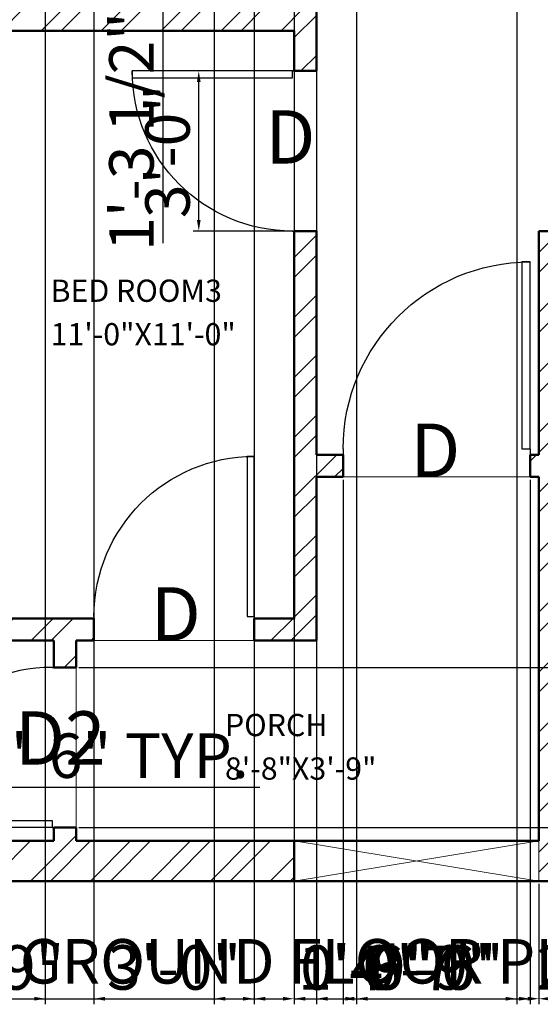
# Model space of a CAD drawing. Units: inches. Extents: x 3824 to 4289, y 1731 to 2259.
# Tile 2 of 5: x 3952 to 4069, y 1731 to 1952. Entities that reach past the tile are written whole.
import ezdxf

# ---------------------------------------------------------------- set-up
doc = ezdxf.new("R2010")
doc.units = ezdxf.units.IN
for name, color, linetype, lineweight in [('A-ANNO-DIMS', 2, 'Continuous', 18), ('A-ANNO-TEXT', 2, 'Continuous', 18), ('A-ANNO-TITL', 2, 'Continuous', 25), ('A-AREA-IDEN', 2, 'Continuous', 18), ('A-FLOR-THRS', 8, 'Continuous', 18), ('DOOR', 6, 'Continuous', 25), ('WALL', 20, 'Continuous', 50)]:
    doc.layers.add(name, color=color, linetype=linetype, lineweight=lineweight)
doc.layers.add('A-WALL-PATT', color=251, linetype='Continuous', lineweight=13, true_color=0x636466)
doc.styles.get("Standard").update_dxf_attribs({"font": 'arial.ttf'})
doc.dimstyles.new('ISO-25', dxfattribs={"dimtxt": 10, "dimasz": 2.5, "dimexe": 1.25, "dimexo": 0.625, "dimtad": 1, "dimdec": 1, "dimlunit": 3, "dimtxsty": 'Standard', "dimcen": 2.5, "dimadec": 0, "dimazin": 0, "dimtfac": 1, "dimtdec": 1, "dimtmove": 0, "dimatfit": 3, "dimfxl": 1, "dimarcsym": 0})

# ---------------------------------------------------------------- blocks, each defined once
blk = doc.blocks.new('*U2')
for p, q in [((0, 0), (0, -6)), ((40, 0), (40, -6))]:
    blk.add_line(p, q)
blk.add_lwpolyline([(0, 0), (0, 40), (1.75, 40), (1.75, 0)], close=True)
blk.add_arc((0, 0), 40, 0, 90)
blk = doc.blocks.new('*D16')
at = {"layer": 'A-ANNO-DIMS', "color": 0, "lineweight": -2, "transparency": 16777216}
for p, q in [((3883.53, 1783.56), (3883.53, 1778.43)), ((3913.57, 1783.56), (3913.57, 1778.43)), ((3886.03, 1779.68), (3911.07, 1779.68)), ((3913.57, 1779.68), (4005.84, 1779.68))]:
    blk.add_line(p, q, dxfattribs=at)
at = {"layer": 'A-ANNO-DIMS', "color": 0, "transparency": 16777216}
for points in [[(3886.03, 1780.1), (3886.03, 1779.27), (3883.53, 1779.68)], [(3911.07, 1780.1), (3911.07, 1779.27), (3913.57, 1779.68)]]:
    blk.add_solid(points, dxfattribs=at)
at = {"layer": 'Defpoints', "color": 0, "transparency": 16777216}
for p in [(3883.53, 1784.19), (3913.57, 1784.19), (3913.57, 1779.68)]:
    blk.add_point(p, dxfattribs=at)
at = {"layer": 'A-ANNO-DIMS', "color": 0, "transparency": 16777216, "insert": (3960.95, 1785.48), "char_height": 10, "attachment_point": 5}
blk.add_mtext('WC 2\'-6" TYP.', dxfattribs=at)
blk = doc.blocks.new('*D38')
at = {"layer": 'A-ANNO-DIMS', "color": 0, "lineweight": -2, "transparency": 16777216}
for p, q in [((3872.55, 1757.99), (3872.55, 1730.92)), ((4013.55, 1757.99), (4013.55, 1730.92)), ((3875.05, 1732.17), (4011.05, 1732.17))]:
    blk.add_line(p, q, dxfattribs=at)
at = {"layer": 'A-ANNO-DIMS', "color": 0, "transparency": 16777216}
for points in [[(3875.05, 1732.59), (3875.05, 1731.75), (3872.55, 1732.17)], [(4011.05, 1732.59), (4011.05, 1731.75), (4013.55, 1732.17)]]:
    blk.add_solid(points, dxfattribs=at)
at = {"layer": 'Defpoints', "color": 0, "transparency": 16777216}
for p in [(3872.55, 1758.62), (4013.55, 1758.62), (4013.55, 1732.17)]:
    blk.add_point(p, dxfattribs=at)
at = {"layer": 'A-ANNO-DIMS', "color": 0, "transparency": 16777216, "insert": (3943.05, 1737.9), "char_height": 10, "attachment_point": 5}
blk.add_mtext('11\'-9"', dxfattribs=at)
blk = doc.blocks.new('*D39')
at = {"layer": 'A-ANNO-DIMS', "color": 0, "lineweight": -2, "transparency": 16777216}
for p, q in [((4013.55, 1757.99), (4013.55, 1730.92)), ((4068.55, 1757.99), (4068.55, 1730.92)), ((4016.05, 1732.17), (4066.05, 1732.17))]:
    blk.add_line(p, q, dxfattribs=at)
at = {"layer": 'A-ANNO-DIMS', "color": 0, "transparency": 16777216}
for points in [[(4016.05, 1732.59), (4016.05, 1731.75), (4013.55, 1732.17)], [(4066.05, 1732.59), (4066.05, 1731.75), (4068.55, 1732.17)]]:
    blk.add_solid(points, dxfattribs=at)
at = {"layer": 'Defpoints', "color": 0, "transparency": 16777216}
for p in [(4013.55, 1758.62), (4068.55, 1758.62), (4068.55, 1732.17)]:
    blk.add_point(p, dxfattribs=at)
at = {"layer": 'A-ANNO-DIMS', "color": 0, "transparency": 16777216, "insert": (4041.05, 1737.79), "char_height": 10, "attachment_point": 5}
blk.add_mtext('4\'-7"', dxfattribs=at)
blk = doc.blocks.new('*D40')
at = {"layer": 'A-ANNO-DIMS', "color": 0, "lineweight": -2, "transparency": 16777216}
for p, q in [((4068.55, 1757.99), (4068.55, 1730.92)), ((4097.55, 1757.99), (4097.55, 1730.92)), ((4071.05, 1732.17), (4095.05, 1732.17))]:
    blk.add_line(p, q, dxfattribs=at)
at = {"layer": 'A-ANNO-DIMS', "color": 0, "transparency": 16777216}
for points in [[(4071.05, 1732.59), (4071.05, 1731.75), (4068.55, 1732.17)], [(4095.05, 1732.59), (4095.05, 1731.75), (4097.55, 1732.17)]]:
    blk.add_solid(points, dxfattribs=at)
at = {"layer": 'Defpoints', "color": 0, "transparency": 16777216}
for p in [(4068.55, 1758.62), (4097.55, 1758.62), (4097.55, 1732.17)]:
    blk.add_point(p, dxfattribs=at)
at = {"layer": 'A-ANNO-DIMS', "color": 0, "transparency": 16777216, "insert": (4083.05, 1737.9), "char_height": 10, "attachment_point": 5}
blk.add_mtext('2\'-5"', dxfattribs=at)
blk = doc.blocks.new('*D42')
at = {"layer": 'A-ANNO-DIMS', "color": 0, "lineweight": -2, "transparency": 16777216}
for p, q in [((4004.55, 2036.99), (4004.55, 1730.92)), ((3968.55, 2031.99), (3968.55, 1730.92)), ((3971.05, 1732.17), (4002.05, 1732.17))]:
    blk.add_line(p, q, dxfattribs=at)
at = {"layer": 'A-ANNO-DIMS', "color": 0, "transparency": 16777216}
for points in [[(3971.05, 1732.59), (3971.05, 1731.75), (3968.55, 1732.17)], [(4002.05, 1732.59), (4002.05, 1731.75), (4004.55, 1732.17)]]:
    blk.add_solid(points, dxfattribs=at)
at = {"layer": 'Defpoints', "color": 0, "transparency": 16777216}
for p in [(4004.55, 2037.62), (3968.55, 2032.62), (4004.55, 1732.17)]:
    blk.add_point(p, dxfattribs=at)
at = {"layer": 'A-ANNO-DIMS', "color": 0, "transparency": 16777216, "insert": (3986.55, 1737.9), "char_height": 10, "attachment_point": 5}
blk.add_mtext('3\'-0"', dxfattribs=at)
blk = doc.blocks.new('*D43')
at = {"layer": 'A-ANNO-DIMS', "color": 0, "lineweight": -2, "transparency": 16777216}
for p, q in [((4004.55, 2036.99), (4004.55, 1730.92)), ((4013.55, 2036.99), (4013.55, 1730.92)), ((4007.05, 1732.17), (4011.05, 1732.17)), ((4013.55, 1732.17), (4043.88, 1732.17))]:
    blk.add_line(p, q, dxfattribs=at)
at = {"layer": 'A-ANNO-DIMS', "color": 0, "transparency": 16777216}
for points in [[(4007.05, 1732.59), (4007.05, 1731.75), (4004.55, 1732.17)], [(4011.05, 1732.59), (4011.05, 1731.75), (4013.55, 1732.17)]]:
    blk.add_solid(points, dxfattribs=at)
at = {"layer": 'Defpoints', "color": 0, "transparency": 16777216}
for p in [(4004.55, 2037.62), (4013.55, 2037.62), (4013.55, 1732.17)]:
    blk.add_point(p, dxfattribs=at)
at = {"layer": 'A-ANNO-DIMS', "color": 0, "transparency": 16777216, "insert": (4029.97, 1737.9), "char_height": 10, "attachment_point": 5}
blk.add_mtext('0\'-9"', dxfattribs=at)
blk = doc.blocks.new('*D44')
at = {"layer": 'A-ANNO-DIMS', "color": 0, "lineweight": -2, "transparency": 16777216}
for p, q in [((4018.55, 2036.99), (4018.55, 1730.92)), ((4027.55, 2031.99), (4027.55, 1730.92)), ((4021.05, 1732.17), (4025.05, 1732.17)), ((4027.55, 1732.17), (4057.88, 1732.17))]:
    blk.add_line(p, q, dxfattribs=at)
at = {"layer": 'A-ANNO-DIMS', "color": 0, "transparency": 16777216}
for points in [[(4021.05, 1732.59), (4021.05, 1731.75), (4018.55, 1732.17)], [(4025.05, 1732.59), (4025.05, 1731.75), (4027.55, 1732.17)]]:
    blk.add_solid(points, dxfattribs=at)
at = {"layer": 'Defpoints', "color": 0, "transparency": 16777216}
for p in [(4018.55, 2037.62), (4027.55, 2032.62), (4027.55, 1732.17)]:
    blk.add_point(p, dxfattribs=at)
at = {"layer": 'A-ANNO-DIMS', "color": 0, "transparency": 16777216, "insert": (4043.97, 1737.9), "char_height": 10, "attachment_point": 5}
blk.add_mtext('0\'-9"', dxfattribs=at)
blk = doc.blocks.new('*D45')
at = {"layer": 'A-ANNO-DIMS', "color": 0, "lineweight": -2, "transparency": 16777216}
for p, q in [((4027.55, 2031.99), (4027.55, 1730.92)), ((4063.55, 2031.99), (4063.55, 1730.92)), ((4030.05, 1732.17), (4061.05, 1732.17))]:
    blk.add_line(p, q, dxfattribs=at)
at = {"layer": 'A-ANNO-DIMS', "color": 0, "transparency": 16777216}
for points in [[(4030.05, 1732.59), (4030.05, 1731.75), (4027.55, 1732.17)], [(4061.05, 1732.59), (4061.05, 1731.75), (4063.55, 1732.17)]]:
    blk.add_solid(points, dxfattribs=at)
at = {"layer": 'Defpoints', "color": 0, "transparency": 16777216}
for p in [(4027.55, 2032.62), (4063.55, 2032.62), (4063.55, 1732.17)]:
    blk.add_point(p, dxfattribs=at)
at = {"layer": 'A-ANNO-DIMS', "color": 0, "transparency": 16777216, "insert": (4045.55, 1737.9), "char_height": 10, "attachment_point": 5}
blk.add_mtext('3\'-0"', dxfattribs=at)
blk = doc.blocks.new('*D46')
at = {"layer": 'A-ANNO-DIMS', "color": 0, "lineweight": -2, "transparency": 16777216}
for p, q in [((4017.93, 1940.62), (3990.85, 1940.62)), ((3992.1, 1907.12), (3992.1, 1938.12)), ((4017.93, 1904.62), (3990.85, 1904.62))]:
    blk.add_line(p, q, dxfattribs=at)
at = {"layer": 'A-ANNO-DIMS', "color": 0, "transparency": 16777216}
for points in [[(3991.69, 1938.12), (3992.52, 1938.12), (3992.1, 1940.62)], [(3991.69, 1907.12), (3992.52, 1907.12), (3992.1, 1904.62)]]:
    blk.add_solid(points, dxfattribs=at)
at = {"layer": 'Defpoints', "color": 0, "transparency": 16777216}
for p in [(3992.1, 1940.62), (4018.55, 1940.62), (4018.55, 1904.62)]:
    blk.add_point(p, dxfattribs=at)
at = {"layer": 'A-ANNO-DIMS', "color": 0, "transparency": 16777216, "insert": (3986.37, 1922.62), "char_height": 10, "attachment_point": 5, "rotation": 90}
blk.add_mtext('3\'-0"', dxfattribs=at)
blk = doc.blocks.new('*D47')
at = {"layer": 'A-ANNO-DIMS', "color": 0, "lineweight": -2, "transparency": 16777216}
for p, q in [((4024.55, 1848.77), (4024.55, 1730.92)), ((4066.55, 1848.77), (4066.55, 1730.92)), ((4027.05, 1732.17), (4064.05, 1732.17))]:
    blk.add_line(p, q, dxfattribs=at)
at = {"layer": 'A-ANNO-DIMS', "color": 0, "transparency": 16777216}
for points in [[(4027.05, 1732.59), (4027.05, 1731.75), (4024.55, 1732.17)], [(4064.05, 1732.59), (4064.05, 1731.75), (4066.55, 1732.17)]]:
    blk.add_solid(points, dxfattribs=at)
at = {"layer": 'Defpoints', "color": 0, "transparency": 16777216}
for p in [(4024.55, 1849.39), (4066.55, 1849.39), (4066.55, 1732.17)]:
    blk.add_point(p, dxfattribs=at)
at = {"layer": 'A-ANNO-DIMS', "color": 0, "transparency": 16777216, "insert": (4045.55, 1737.9), "char_height": 10, "attachment_point": 5}
blk.add_mtext('3\'-6"', dxfattribs=at)
blk = doc.blocks.new('*D48')
at = {"layer": 'A-ANNO-DIMS', "color": 0, "lineweight": -2, "transparency": 16777216}
for p, q in [((3968.55, 1811.99), (3968.55, 1730.92)), ((4004.55, 1811.99), (4004.55, 1730.92)), ((3971.05, 1732.17), (4002.05, 1732.17))]:
    blk.add_line(p, q, dxfattribs=at)
at = {"layer": 'A-ANNO-DIMS', "color": 0, "transparency": 16777216}
for points in [[(3971.05, 1732.59), (3971.05, 1731.75), (3968.55, 1732.17)], [(4002.05, 1732.59), (4002.05, 1731.75), (4004.55, 1732.17)]]:
    blk.add_solid(points, dxfattribs=at)
at = {"layer": 'Defpoints', "color": 0, "transparency": 16777216}
for p in [(3968.55, 1812.62), (4004.55, 1812.62), (4004.55, 1732.17)]:
    blk.add_point(p, dxfattribs=at)
at = {"layer": 'A-ANNO-DIMS', "color": 0, "transparency": 16777216, "insert": (3986.55, 1737.9), "char_height": 10, "attachment_point": 5}
blk.add_mtext('3\'-0"', dxfattribs=at)
blk = doc.blocks.new('*D49')
at = {"layer": 'A-ANNO-DIMS', "color": 0, "lineweight": -2, "transparency": 16777216}
for p, q in [((3965.18, 1806.62), (4188.25, 1806.62)), ((4187, 1773.12), (4187, 1804.12)), ((3965.18, 1770.62), (4188.25, 1770.62))]:
    blk.add_line(p, q, dxfattribs=at)
at = {"layer": 'A-ANNO-DIMS', "color": 0, "transparency": 16777216}
for points in [[(4186.59, 1804.12), (4187.42, 1804.12), (4187, 1806.62)], [(4186.59, 1773.12), (4187.42, 1773.12), (4187, 1770.62)]]:
    blk.add_solid(points, dxfattribs=at)
at = {"layer": 'Defpoints', "color": 0, "transparency": 16777216}
for p in [(3964.55, 1806.62), (4187, 1806.62), (3964.55, 1770.62)]:
    blk.add_point(p, dxfattribs=at)
at = {"layer": 'A-ANNO-DIMS', "color": 0, "transparency": 16777216, "insert": (4181.27, 1788.62), "char_height": 10, "attachment_point": 5, "rotation": 90}
blk.add_mtext('3\'-0"', dxfattribs=at)
blk = doc.blocks.new('*D56')
at = {"layer": 'A-ANNO-DIMS', "color": 0, "lineweight": -2, "transparency": 16777216}
for p, q in [((3995.55, 2120.99), (3995.55, 1730.92)), ((4013.55, 2120.99), (4013.55, 1730.92)), ((3998.05, 1732.17), (4011.05, 1732.17)), ((4013.55, 1732.17), (4042.94, 1732.17))]:
    blk.add_line(p, q, dxfattribs=at)
at = {"layer": 'A-ANNO-DIMS', "color": 0, "transparency": 16777216}
for points in [[(3998.05, 1732.59), (3998.05, 1731.75), (3995.55, 1732.17)], [(4011.05, 1732.59), (4011.05, 1731.75), (4013.55, 1732.17)]]:
    blk.add_solid(points, dxfattribs=at)
at = {"layer": 'Defpoints', "color": 0, "transparency": 16777216}
for p in [(3995.55, 2121.62), (4013.55, 2121.62), (4013.55, 1732.17)]:
    blk.add_point(p, dxfattribs=at)
at = {"layer": 'A-ANNO-DIMS', "color": 0, "transparency": 16777216, "insert": (4029.5, 1737.9), "char_height": 10, "attachment_point": 5}
blk.add_mtext('1\'-6"', dxfattribs=at)
blk = doc.blocks.new('*D58')
at = {"layer": 'A-ANNO-DIMS', "color": 0, "lineweight": -2, "transparency": 16777216}
for p, q in [((3881.55, 1953.99), (3881.55, 1730.92)), ((3957.61, 1953.99), (3957.61, 1730.92)), ((3884.05, 1732.17), (3955.11, 1732.17))]:
    blk.add_line(p, q, dxfattribs=at)
at = {"layer": 'A-ANNO-DIMS', "color": 0, "transparency": 16777216}
for points in [[(3884.05, 1732.59), (3884.05, 1731.75), (3881.55, 1732.17)], [(3955.11, 1732.59), (3955.11, 1731.75), (3957.61, 1732.17)]]:
    blk.add_solid(points, dxfattribs=at)
at = {"layer": 'Defpoints', "color": 0, "transparency": 16777216}
for p in [(3881.55, 1954.62), (3957.61, 1954.62), (3957.61, 1732.17)]:
    blk.add_point(p, dxfattribs=at)
at = {"layer": 'A-ANNO-DIMS', "color": 0, "transparency": 16777216, "insert": (3919.58, 1737.9), "char_height": 10, "attachment_point": 5}
blk.add_mtext('6\'-4"', dxfattribs=at)
blk = doc.blocks.new('*D61')
at = {"layer": 'A-ANNO-DIMS', "color": 0, "lineweight": -2, "transparency": 16777216}
for p, q in [((3958.23, 1970.11), (3985.31, 1970.11)), ((3984.06, 1967.61), (3984.06, 1957.12)), ((3958.23, 1954.62), (3985.31, 1954.62)), ((3984.06, 1954.62), (3984.06, 1901.93))]:
    blk.add_line(p, q, dxfattribs=at)
at = {"layer": 'A-ANNO-DIMS', "color": 0, "transparency": 16777216}
for points in [[(3983.64, 1967.61), (3984.47, 1967.61), (3984.06, 1970.11)], [(3983.64, 1957.12), (3984.47, 1957.12), (3984.06, 1954.62)]]:
    blk.add_solid(points, dxfattribs=at)
at = {"layer": 'Defpoints', "color": 0, "transparency": 16777216}
for p in [(3957.61, 1970.11), (3957.61, 1954.62), (3984.06, 1954.62)]:
    blk.add_point(p, dxfattribs=at)
at = {"layer": 'A-ANNO-DIMS', "color": 0, "transparency": 16777216, "insert": (3978.26, 1927.02), "char_height": 10, "attachment_point": 5, "rotation": 90}
blk.add_mtext('1\'-3 1/2"', dxfattribs=at)

msp = doc.modelspace()

# ---------------------------------------------------------------- hatches: boundary and pattern name
at = {"layer": 'A-WALL-PATT'}
h = msp.add_hatch(dxfattribs=at)
h.set_pattern_fill('ANSI32', color=256)
h.paths.add_polyline_path([(4018.55, 1954.62), (3881.55, 1954.62), (3881.55, 1969.62), (3872.55, 1969.62), (3872.55, 1901.62), (3881.53, 1901.62), (3881.53, 1903.2, -0.148069), (3880.67, 1906.03, -0.148069), (3881.53, 1908.87), (3881.53, 1910.29), (3881.55, 1949.62), (4013.55, 1949.62), (4013.55, 1940.62), (4018.55, 1940.62)])
h = msp.add_hatch(dxfattribs=at)
h.set_pattern_fill('ANSI32', color=256)
h.paths.add_polyline_path([(4018.55, 1904.62), (4013.55, 1904.62), (4013.55, 1817.62), (4004.55, 1817.62), (4004.55, 1812.62), (4018.55, 1812.62), (4018.55, 1849.39), (4024.55, 1849.39), (4024.55, 1854.39), (4018.55, 1854.39)])
h = msp.add_hatch(dxfattribs=at)
h.set_pattern_fill('ANSI32', color=256)
h.paths.add_polyline_path([(4073.55, 1904.62), (4068.55, 1904.62), (4068.55, 1854.39), (4066.55, 1854.39), (4066.55, 1849.39), (4068.55, 1849.39), (4068.55, 1767.62), (4068.55, 1758.62), (4097.55, 1758.62), (4097.55, 1767.62), (4073.55, 1767.62), (4073.55, 1812.62), (4079.55, 1812.62), (4079.55, 1817.62), (4073.55, 1817.62)])
h = msp.add_hatch(dxfattribs=at)
h.set_pattern_fill('ANSI32', color=256)
h.paths.add_polyline_path([(3881.55, 1812.62), (3959.55, 1812.62), (3959.55, 1806.62), (3964.55, 1806.62), (3964.55, 1812.62), (3968.55, 1812.62), (3968.55, 1817.62), (3881.55, 1817.62), (3881.55, 1831.44), (3881.53, 1831.44), (3881.53, 1832.85, -0.148069), (3880.67, 1835.69, -0.148069), (3881.53, 1838.52), (3881.53, 1844.19), (3881.53, 1853.62), (3872.55, 1853.62), (3872.55, 1803.62), (3881.55, 1803.62)])
h = msp.add_hatch(dxfattribs=at)
h.set_pattern_fill('ANSI32', color=256)
h.paths.add_polyline_path([(4013.55, 1767.62), (3964.55, 1767.62), (3964.55, 1770.62), (3959.55, 1770.62), (3959.55, 1767.62), (3881.55, 1767.62), (3881.55, 1779.62), (3872.55, 1779.62), (3872.55, 1758.62), (4013.55, 1758.62)])

# ---------------------------------------------------------------- linework, layer by layer
at = {"layer": 'A-FLOR-THRS'}
for p, q in [((4018.55, 1940.62), (4018.55, 1904.62)), ((4024.55, 1849.39), (4066.55, 1849.39)), ((3968.55, 1812.62), (4004.55, 1812.62)), ((3964.55, 1806.62), (3964.55, 1770.62)), ((4013.55, 1758.62), (4068.55, 1767.62)), ((4068.55, 1758.62), (4013.55, 1767.62))]:
    msp.add_line(p, q, dxfattribs=at)
msp.add_lwpolyline([(4013.55, 1767.62), (4068.55, 1767.62), (4068.55, 1758.62), (4013.55, 1758.62)], close=True, dxfattribs=at)
at = {"layer": 'WALL'}
for p, q in [((4018.55, 1954.62), (4018.55, 1940.62)), ((3881.55, 1949.62), (4013.55, 1949.62)), ((4013.55, 1949.62), (4013.55, 1940.62)), ((4013.55, 1940.62), (4018.55, 1940.62)), ((4013.55, 1904.62), (4018.55, 1904.62)), ((4013.55, 1904.62), (4013.55, 1817.62)), ((4018.55, 1904.62), (4018.55, 1854.39)), ((4068.55, 1904.62), (4068.55, 1854.39)), ((4068.55, 1904.62), (4073.55, 1904.62)), ((4018.55, 1854.39), (4024.55, 1854.39)), ((4024.55, 1849.39), (4024.55, 1854.39)), ((4066.55, 1849.39), (4066.55, 1854.39)), ((4066.55, 1854.39), (4068.55, 1854.39)), ((4018.55, 1849.39), (4024.55, 1849.39)), ((4018.55, 1849.39), (4018.55, 1812.62)), ((4066.55, 1849.39), (4068.55, 1849.39)), ((4068.55, 1849.39), (4068.55, 1767.62)), ((3881.55, 1817.62), (3968.55, 1817.62)), ((3968.55, 1817.62), (3968.55, 1812.62)), ((4004.55, 1817.62), (4004.55, 1812.62)), ((4004.55, 1817.62), (4013.55, 1817.62)), ((3881.55, 1812.62), (3959.55, 1812.62)), ((3959.55, 1812.62), (3959.55, 1806.62)), ((3964.55, 1812.62), (3964.55, 1806.62)), ((3964.55, 1812.62), (3968.55, 1812.62)), ((4004.55, 1812.62), (4018.55, 1812.62)), ((3964.55, 1806.62), (3959.55, 1806.62)), ((3964.55, 1770.62), (3959.55, 1770.62)), ((3959.55, 1770.62), (3959.55, 1767.62)), ((3964.55, 1770.62), (3964.55, 1767.62)), ((3881.55, 1767.62), (3959.55, 1767.62)), ((3964.55, 1767.62), (4013.55, 1767.62)), ((4013.55, 1767.62), (4013.55, 1758.62)), ((4013.55, 1767.62), (4068.55, 1767.62)), ((3872.55, 1758.62), (4013.55, 1758.62)), ((4013.55, 1758.62), (4160.55, 1758.62))]:
    msp.add_line(p, q, dxfattribs=at)

# ---------------------------------------------------------------- block references
at = {"layer": 'DOOR'}
for p, xscale, yscale, zscale, rotation in [((4013.15, 1940.62), -0.9, 0.9, 0.9, 90), ((3959.15, 1770.62), 0.9000000000000028, 0.9000000000000028, 0.9000000000000028, 90.00000000000003)]:
    msp.add_blockref('*U2', p, dxfattribs=dict(at, xscale=xscale, yscale=yscale, zscale=zscale, rotation=rotation))
for p, xscale, yscale, zscale in [((4066.55, 1855.69), -1.049999999999988, 1.049999999999988, 1.049999999999988), ((4004.55, 1818.02), -0.9, 0.9, 0.9)]:
    msp.add_blockref('*U2', p, dxfattribs=dict(at, xscale=xscale, yscale=yscale, zscale=zscale))

# ---------------------------------------------------------------- texts
at = {"layer": 'A-ANNO-TEXT'}
for s, p in [('D', (4007.06, 1919.78)), ('D', (4039.62, 1849.39)), ('D', (3981.3, 1812.62)), ('D2', (3950.8, 1784.74))]:
    msp.add_text(s, height=12, dxfattribs=at).set_placement(p)
at = {"layer": 'A-ANNO-TITL'}
msp.add_text('GROUND FLOOR PLAN', height=10, dxfattribs=at).set_placement((3951.87, 1735.58))
at = {"layer": 'A-AREA-IDEN'}
for s, p in [('BED ROOM3', (3958.8, 1888.73)), ('11\'-0"X11\'-0"', (3958.8, 1878.95)), ('PORCH', (3997.99, 1791.16)), ('8\'-8"X3\'-9"', (3997.99, 1781.38))]:
    msp.add_text(s, height=5, dxfattribs=at).set_placement(p)

# ---------------------------------------------------------------- dimensions: what is measured, and where the dimension line sits
at = {"layer": 'A-ANNO-DIMS'}
for base, p1, p2, picture, middle in [((4013.55, 1732.17), (3995.55, 2121.62), (4013.55, 2121.62), '*D56', (4029.5, 1737.9)), ((4004.55, 1732.17), (3968.55, 2032.62), (4004.55, 2037.62), '*D42', (3986.55, 1737.9)), ((4013.55, 1732.17), (4004.55, 2037.62), (4013.55, 2037.62), '*D43', (4029.97, 1737.9)), ((4027.55, 1732.17), (4018.55, 2037.62), (4027.55, 2032.62), '*D44', (4043.97, 1737.9)), ((4063.55, 1732.17), (4027.55, 2032.62), (4063.55, 2032.62), '*D45', (4045.55, 1737.9)), ((3957.61, 1732.17), (3881.55, 1954.62), (3957.61, 1954.62), '*D58', (3919.58, 1737.9)), ((4066.55, 1732.17), (4024.55, 1849.39), (4066.55, 1849.39), '*D47', (4045.55, 1737.9)), ((4004.55, 1732.17), (3968.55, 1812.62), (4004.55, 1812.62), '*D48', (3986.55, 1737.9)), ((4013.55, 1732.17), (3872.55, 1758.62), (4013.55, 1758.62), '*D38', (3943.05, 1737.9)), ((4068.55, 1732.17), (4013.55, 1758.62), (4068.55, 1758.62), '*D39', (4041.05, 1737.79)), ((4097.55, 1732.17), (4068.55, 1758.62), (4097.55, 1758.62), '*D40', (4083.05, 1737.9))]:
    dim = msp.add_linear_dim(base=base, p1=p1, p2=p2, dimstyle='ISO-25', override={"dimdec": 1, "dimlfac": 1, "dimrnd": 0, "dimzin": 1, "dimdsep": 46, "dimlunit": 4, "dimfrac": 2}, dxfattribs=at)
    dim.commit()
    dim.dimension.update_dxf_attribs({"geometry": picture, "text_midpoint": middle})
for base, p1, p2, angle, picture, middle in [((3984.06, 1954.62), (3957.61, 1970.11), (3957.61, 1954.62), 270, '*D61', (3978.26, 1927.02)), ((3992.1, 1940.62), (4018.55, 1904.62), (4018.55, 1940.62), 90, '*D46', (3986.37, 1922.62)), ((4187, 1806.62), (3964.55, 1770.62), (3964.55, 1806.62), 90, '*D49', (4181.27, 1788.62))]:
    dim = msp.add_linear_dim(base=base, p1=p1, p2=p2, angle=angle, dimstyle='ISO-25', override={"dimdec": 1, "dimlfac": 1, "dimrnd": 0, "dimzin": 1, "dimdsep": 46, "dimlunit": 4, "dimfrac": 2}, dxfattribs=at)
    dim.commit()
    dim.dimension.update_dxf_attribs({"geometry": picture, "text_midpoint": middle})
dim = msp.add_linear_dim(base=(3913.57, 1779.68), p1=(3883.53, 1784.19), p2=(3913.57, 1784.19), text='WC <> TYP.', dimstyle='ISO-25', override={"dimdec": 1, "dimlfac": 1, "dimrnd": 0, "dimzin": 1, "dimdsep": 46, "dimlunit": 4, "dimfrac": 2}, dxfattribs=at)
dim.commit()
dim.dimension.update_dxf_attribs({"geometry": '*D16', "text_midpoint": (3960.95, 1785.48)})

doc.saveas('drawing.dxf')
